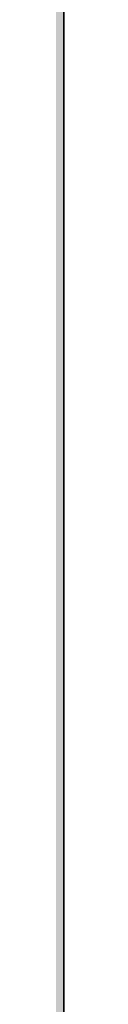
# Model space of a CAD drawing. Units: inches. Extents: x 2091 to 2899, y 967 to 2217.
# Tile 65 of 256: x 2212.1436 to 2212.1436, y 1100.4988 to 1101.1654. Entities that reach past the tile are written whole.
import ezdxf

# ---------------------------------------------------------------- set-up
doc = ezdxf.new("R2010")
doc.units = ezdxf.units.IN
doc.layers.add('A-WALL', color=7, linetype='Continuous', lineweight=35)
doc.layers.add('A-WALL-PATT', color=141, linetype='Continuous', lineweight=13, true_color=0xadddf7)

msp = doc.modelspace()

# ---------------------------------------------------------------- hatches: boundary and pattern name
at = {"layer": 'A-WALL-PATT'}
h = msp.add_hatch(color=256, dxfattribs=at)
h.dxf.hatch_style = 1
h.paths.add_polyline_path([(2212.1436, 1941.41906), (2387.6436, 1941.41906), (2387.6436, 1824.41906), (2392.1436, 1824.41906), (2392.1436, 1941.41906), (2609.6436, 1941.41906), (2609.6436, 1825.91906), (2614.1436, 1825.91906), (2614.1436, 1941.41906), (2794.1436, 1941.41906), (2794.1436, 1928.76217), (2803.1436, 1928.76217), (2803.1436, 2050.91906), (2203.1436, 2050.91906), (2203.1436, 1900.75786), (2212.1436, 1900.75786)])
h.paths.add_polyline_path([(2212.1436, 1945.91906), (2212.1436, 2041.91906), (2794.1436, 2041.91906), (2794.1436, 1945.91906), (2402.24824, 1945.91906), (2401.10243, 1945.77583), (2398.70243, 1945.77583)], flags=16)
h.paths.add_polyline_path([(2230.22986, 1948.06279), (2227.34986, 1949.50279), (2225.90986, 1951.90279), (2223.98986, 1952.86279), (2223.02986, 1955.26279), (2222.06986, 1959.58279), (2222.06986, 1963.42279), (2223.02986, 1965.66279), (2223.98986, 1965.34279), (2225.58591, 1963.86075), (2226.91153, 1964.95726), (2226.94886, 1965.93879), (2227.77832, 1966.95214), (2228.19992, 1968.8787), (2230.70986, 1964.86279), (2233.58986, 1966.30279), (2233.60731, 1966.33187), (2233.77266, 1964.9382), (2234.6338, 1963.67647), (2235.02986, 1963.90279), (2236.28203, 1965.57236), (2235.98986, 1962.94279), (2237.95451, 1957.54), (2238.38986, 1957.90279), (2239.21586, 1960.30579), (2238.65457, 1966.38496), (2238.69279, 1966.43807), (2238.84058, 1967.49971), (2238.78029, 1967.68749), (2238.88054, 1967.78676), (2238.66686, 1966.25179), (2239.21586, 1960.30579), (2238.38986, 1957.90279), (2236.94986, 1956.70279), (2234.54986, 1949.98279)], flags=0)
h.paths.add_polyline_path([(2278.01197, 1948.06279), (2276.49643, 1947.87335), (2275.84983, 1947.68861), (2274.65197, 1947.10279)], flags=0)
h.paths.add_polyline_path([(2269.85197, 1955.74279), (2268.27618, 1956.62933), (2270.8673, 1956.3484), (2269.37197, 1958.14279), (2268.71496, 1959.19233), (2270.56983, 1958.72861), (2268.58073, 1961.90609), (2270.81197, 1960.89188), (2270.81197, 1963.42279), (2271.39331, 1964.77926), (2270.29176, 1966.1562), (2271.77197, 1965.66279), (2272.14139, 1966.52476), (2273.92983, 1965.92861), (2275.63039, 1968.0543), (2276.33194, 1966.72186), (2276.52043, 1966.95214), (2276.94203, 1968.8787), (2277.73429, 1967.61108), (2278.13989, 1969.46452), (2279.65912, 1967.03374), (2280.41197, 1966.78279), (2280.9493, 1967.58879), (2281.60983, 1967.36861), (2282.13327, 1968.15376), (2282.34924, 1966.33344), (2282.34985, 1966.33259), (2283.40755, 1968.09542), (2283.71263, 1965.52402), (2284.32022, 1964.63379), (2284.51181, 1964.88924), (2284.23497, 1965.70479), (2284.50047, 1967.31896), (2284.90794, 1965.41742), (2285.39631, 1966.06858), (2285.43283, 1966.29061), (2285.47334, 1966.17128), (2286.35392, 1967.34539), (2286.22201, 1966.15817), (2287.66349, 1968.08015), (2287.71397, 1968.44279), (2288.4816, 1969.01668), (2288.57399, 1968.7289), (2288.91746, 1969.06904), (2288.60683, 1966.83761), (2288.92873, 1963.35131), (2288.93497, 1963.35679), (2288.92973, 1963.34042), (2289.01528, 1962.41387), (2290.11122, 1963.87513), (2290.13283, 1963.94261), (2290.21767, 1964.01706), (2290.11122, 1963.87513), (2289.15583, 1960.89161), (2288.59404, 1959.25723), (2288.57197, 1959.10279), (2289.53197, 1960.54279), (2290.01197, 1962.46279), (2290.19184, 1962.64266), (2289.76983, 1959.68861), (2286.88983, 1957.28861), (2284.48983, 1950.56861), (2283.31466, 1950.04631), (2283.29197, 1949.98279), (2280.29006, 1948.64861), (2281.12983, 1948.64861), (2282.56983, 1948.16861), (2283.20473, 1948.06279), (2278.97197, 1948.06279), (2276.09197, 1949.50279), (2274.65197, 1951.90279), (2272.73197, 1952.86279)], flags=0)
h.paths.add_polyline_path([(2271.15887, 1958.02177), (2272.96983, 1955.84861), (2272.00983, 1960.16861), (2272.00983, 1964.00861), (2272.62443, 1965.44266), (2274.32802, 1963.86075), (2275.65365, 1964.95726), (2275.63774, 1964.53909), (2277.41223, 1966.00689), (2277.03297, 1965.15679), (2276.82992, 1964.9756), (2276.76601, 1963.29501), (2277.44964, 1962.66022), (2279.45197, 1964.86279), (2282.33197, 1966.30279), (2283.52983, 1966.88861), (2283.29451, 1966.77095), (2283.91299, 1963.8847), (2284.89925, 1964.44827), (2284.73197, 1962.94279), (2286.69662, 1957.54), (2287.13197, 1957.90279), (2287.54191, 1959.09539), (2287.7794, 1958.44231), (2285.68274, 1956.6951), (2285.8765, 1959.79534), (2284.73197, 1962.94279), (2284.89925, 1964.44827), (2283.91299, 1963.8847), (2284.22383, 1962.43412), (2283.42436, 1963.60548), (2281.60983, 1962.56861), (2281.12983, 1960.16861), (2282.08983, 1956.32861), (2283.04983, 1952.96861), (2282.56983, 1950.56861), (2280.16983, 1948.64861), (2279.88332, 1948.79187), (2278.97197, 1948.06279), (2278.97197, 1949.02279), (2278.67231, 1949.39737), (2277.28983, 1950.08861), (2275.84983, 1952.48861), (2273.92983, 1953.44861), (2272.48983, 1954.88861), (2271.92165, 1954.88861), (2271.77197, 1955.26279)], flags=0)
h.paths.add_polyline_path([(2311.99415, 1955.74279), (2312.06272, 1955.67422), (2312.0551, 1955.7085)], flags=0)
h.paths.add_polyline_path([(2331.95615, 1963.95179), (2333.39615, 1965.39179), (2331.07715, 1963.35679), (2330.9986, 1963.11152)], flags=0)
h.paths.add_polyline_path([(2310.55415, 1954.30279), (2307.03981, 1956.27994), (2310.7629, 1955.87628), (2312.47415, 1953.82279), (2313.43415, 1951.42279), (2315.35415, 1950.46279), (2316.79415, 1948.06279), (2317.46615, 1947.72679), (2319.36869, 1947.96461), (2317.75415, 1949.98279), (2317.56953, 1950.61048), (2316.79415, 1951.90279), (2314.87415, 1952.86279), (2313.91415, 1955.26279), (2311.51415, 1958.14279), (2309.37549, 1961.55917), (2311.51415, 1960.33708), (2311.51415, 1961.98279), (2310.60467, 1963.11963), (2311.72661, 1962.47853), (2312.41833, 1964.09256), (2312.25596, 1964.29552), (2313.19415, 1963.98279), (2313.91415, 1965.66279), (2314.64678, 1965.41858), (2315.35415, 1966.30279), (2316.79415, 1967.74279), (2316.15744, 1966.9469), (2317.03411, 1965.28186), (2317.2226, 1965.51214), (2317.77705, 1968.04577), (2318.47411, 1966.72186), (2318.6626, 1966.95214), (2319.0842, 1968.8787), (2321.20705, 1965.48215), (2322.16142, 1966.9137), (2322.55415, 1966.78279), (2322.78599, 1967.13056), (2322.88165, 1966.32429), (2323.31204, 1965.72174), (2323.65129, 1965.89136), (2324.3965, 1967.13338), (2324.65694, 1964.9382), (2324.97199, 1964.47661), (2325.38728, 1967.0015), (2325.94081, 1964.41835), (2327.22893, 1966.13584), (2327.16632, 1965.57236), (2328.05914, 1966.76278), (2328.22458, 1966.24749), (2329.66797, 1967.67691), (2329.66458, 1967.68749), (2329.76482, 1967.78676), (2329.55115, 1966.25179), (2330.10015, 1960.30579), (2329.33281, 1958.07347), (2329.31306, 1957.93523), (2329.63415, 1958.20279), (2330.23415, 1959.10279), (2330.71415, 1961.02279), (2331.03415, 1961.34279), (2330.71415, 1959.10279), (2329.63415, 1958.20279), (2329.27415, 1957.66279), (2327.71211, 1956.3611), (2325.43415, 1949.98279), (2324.33377, 1949.49374), (2323.99415, 1948.54279), (2319.67415, 1946.62279), (2316.79415, 1948.06279), (2315.35415, 1950.46279), (2313.43415, 1951.42279)], flags=0)
h.paths.add_polyline_path([(2321.33568, 1947.95202), (2321.11415, 1948.06279), (2321.11415, 1949.02279), (2319.19415, 1951.42279), (2316.79415, 1959.58279), (2316.66324, 1959.58279), (2315.35415, 1958.14279), (2314.39415, 1958.14279), (2313.1483, 1958.70908), (2312.95415, 1959.58279), (2312.95415, 1960.89188), (2315.83415, 1959.58279), (2316.66324, 1959.58279), (2317.31471, 1960.29941), (2315.0302, 1962.42075), (2316.35582, 1963.51726), (2316.37234, 1963.95162), (2316.4702, 1963.86075), (2317.79582, 1964.95726), (2317.75522, 1963.88969), (2319.17515, 1965.15679), (2319.49841, 1965.88137), (2321.11415, 1965.34279), (2323.23589, 1962.37236), (2325.68635, 1963.77262), (2325.54279, 1962.48058), (2325.19878, 1963.49401), (2324.47851, 1963.08243), (2324.92601, 1960.99412), (2324.07809, 1962.23647), (2322.41479, 1961.28602), (2322.07415, 1959.58279), (2323.03415, 1955.74279), (2323.99415, 1952.38279), (2323.51415, 1949.98279), (2322.14272, 1948.88565), (2322.07415, 1948.54279)], flags=0)
h.paths.add_polyline_path([(2320.20748, 1963.33746), (2320.15415, 1963.42279), (2320.39415, 1963.54279)], flags=0)
h.paths.add_polyline_path([(2353.85053, 1965.8105), (2354.03053, 1965.7505), (2354.33053, 1966.4505), (2354.33053, 1966.9305)], flags=0)
h.paths.add_polyline_path([(2359.02058, 1969.02641), (2359.09838, 1968.90193), (2359.23353, 1969.5195), (2359.23353, 1969.9995)], flags=0)
h.paths.add_polyline_path([(2358.25669, 1966.68167), (2357.9836, 1966.34803), (2358.21127, 1966.14617), (2358.41049, 1966.38957)], flags=0)
h.paths.add_polyline_path([(2357.76847, 1966.05878), (2357.7322, 1965.10497), (2357.75105, 1965.12056), (2357.76953, 1965.6065), (2357.76953, 1966.05784)], flags=0)
h.paths.add_polyline_path([(2359.11153, 1965.3045), (2359.11153, 1964.8245), (2359.84453, 1966.4675), (2359.84453, 1966.9475)], flags=0)
h.paths.add_polyline_path([(2360.22368, 1966.62145), (2360.69853, 1969.3625), (2360.69853, 1969.8425), (2360.21053, 1967.0255), (2360.21053, 1966.6425)], flags=0)
h.paths.add_polyline_path([(2363.45053, 1967.8905), (2363.45053, 1968.3705), (2362.49053, 1966.9305), (2362.65604, 1966.69878)], flags=0)
h.paths.add_polyline_path([(2364.47552, 1966.07883), (2365.85053, 1968.3705), (2365.85053, 1968.8505), (2364.42798, 1966.47958)], flags=0)
h.paths.add_polyline_path([(2366.31353, 1965.8525), (2366.36671, 1965.69583), (2366.80253, 1968.3455), (2366.80253, 1968.8255)], flags=0)
h.paths.add_polyline_path([(2367.16531, 1965.80354), (2367.29053, 1966.9305), (2367.29053, 1967.4105), (2367.1027, 1965.72007)], flags=0)
h.paths.add_polyline_path([(2370.03653, 1959.9735), (2371.01353, 1963.0245), (2371.01353, 1963.5045), (2370.03653, 1960.4535)], flags=0)
h.paths.add_polyline_path([(2371.61053, 1960.2105), (2372.57053, 1961.6505), (2372.57053, 1962.1305), (2371.80253, 1960.9785)], flags=0)
h.paths.add_polyline_path([(2350.87367, 1956.00509), (2351.93053, 1955.8905), (2354.49053, 1953.3305), (2353.85053, 1954.9305), (2351.45053, 1957.8105), (2347.93553, 1963.4255), (2347.93553, 1963.9055), (2351.45053, 1958.2905), (2353.70507, 1955.58505), (2352.89053, 1959.2505), (2352.89053, 1959.7305), (2352.89053, 1961.92479), (2356.73053, 1959.7305), (2358.45447, 1961.62684), (2354.81053, 1965.0105), (2355.03086, 1965.28591), (2358.69109, 1961.88712), (2361.53053, 1965.0105), (2364.3765, 1966.43348), (2364.52439, 1965.18691), (2365.45447, 1963.82418), (2365.88107, 1964.06795), (2365.37053, 1966.4505), (2365.37053, 1966.9305), (2366.81053, 1960.2105), (2366.81053, 1959.7305), (2366.38871, 1952.98141), (2367.77053, 1956.8505), (2368.64123, 1957.57608), (2366.81053, 1962.6105), (2366.81053, 1963.0905), (2368.77518, 1957.68771), (2369.21053, 1958.0505), (2370.00159, 1960.35187), (2369.47523, 1966.05267), (2369.51346, 1966.10578), (2369.51417, 1966.11091), (2369.47523, 1966.53267), (2369.51346, 1966.58578), (2369.61463, 1967.31259), (2369.18253, 1968.6585), (2369.18253, 1969.1385), (2369.60096, 1967.83519), (2369.7012, 1967.93447), (2369.71795, 1968.05474), (2370.14518, 1968.37414), (2369.77871, 1968.01122), (2369.7012, 1967.45447), (2370.46816, 1968.214), (2369.67494, 1967.26577), (2369.51417, 1966.11091), (2370.03653, 1960.4535), (2370.03653, 1959.9735), (2369.44176, 1958.24319), (2370.65053, 1959.2505), (2371.04582, 1962.01756), (2371.13053, 1962.1305), (2370.65053, 1958.7705), (2367.77053, 1956.3705), (2365.37053, 1949.6505), (2362.0791, 1948.18764), (2363.45053, 1947.7305), (2361.05053, 1947.7305), (2360.09053, 1947.7305), (2357.10386, 1947.35717), (2360.09053, 1948.2105), (2358.17053, 1949.1705), (2356.73053, 1951.5705), (2354.81053, 1952.5305), (2351.93053, 1955.4105)], flags=0)
h.paths.add_polyline_path([(2361.05053, 1948.6905), (2359.13053, 1951.0905), (2356.73053, 1959.2505), (2355.77053, 1959.2505), (2352.89053, 1960.55959), (2352.89053, 1961.44479), (2355.89053, 1959.7305), (2356.73053, 1959.7305), (2356.83719, 1959.36783), (2361.53053, 1964.5305), (2363.24842, 1965.38945), (2364.92531, 1963.0418), (2362.49053, 1961.6505), (2362.06386, 1959.51717), (2362.97053, 1955.8905), (2363.93053, 1952.5305), (2363.93053, 1952.0505), (2363.45053, 1949.6505), (2361.05053, 1947.7305)], flags=0)
h.paths.add_polyline_path([(2359.13053, 1951.5705), (2359.29053, 1951.3705), (2361.05053, 1954.4505), (2361.05053, 1954.9305)], flags=0)
h.paths.add_polyline_path([(2357.21953, 1966.5455), (2356.79253, 1968.8145), (2356.79253, 1969.2945), (2357.21953, 1967.0255)], flags=0)
h.paths.add_polyline_path([(2361.05053, 1954.4505), (2361.53053, 1958.7705), (2361.53053, 1959.2505), (2361.05053, 1954.9305)], flags=0)
h.paths.add_polyline_path([(2402.54829, 1948.48608), (2402.30243, 1948.41583), (2402.59043, 1948.41583)], flags=0)
h.paths.add_polyline_path([(2394.14243, 1956.09583), (2395.68505, 1954.55321), (2396.7205, 1953.97068), (2396.06243, 1955.61583), (2395.24138, 1956.6011), (2395.8789, 1956.44171), (2395.10243, 1959.93583), (2395.10243, 1963.77583), (2396.06243, 1966.01583), (2397.02243, 1965.69583), (2398.61848, 1964.21379), (2399.94411, 1965.3103), (2399.98143, 1966.29183), (2400.81089, 1967.30518), (2401.23249, 1969.23174), (2403.53795, 1965.54301), (2403.94198, 1967.38932), (2404.70243, 1967.13583), (2405.46033, 1966.07478), (2406.62243, 1966.65583), (2406.63988, 1966.68491), (2406.80523, 1965.29124), (2406.92569, 1965.11475), (2407.34243, 1964.97583), (2407.87433, 1965.77367), (2408.1691, 1964.39805), (2409.31461, 1965.9254), (2409.21746, 1965.05105), (2409.44523, 1963.13124), (2410.30637, 1961.86951), (2410.70243, 1962.09583), (2411.44227, 1963.08228), (2411.16543, 1963.89783), (2411.61643, 1966.63976), (2411.72536, 1966.79111), (2411.87315, 1967.85275), (2411.81286, 1968.04053), (2411.91311, 1968.1398), (2411.69943, 1966.60483), (2412.24843, 1960.65883), (2413.22543, 1963.70983), (2414.3779, 1964.72116), (2414.51315, 1965.69275), (2414.45286, 1965.88053), (2414.55311, 1965.9798), (2414.3779, 1964.72116), (2414.51982, 1964.8457), (2414.36536, 1964.63111), (2414.33943, 1964.44483), (2414.88843, 1958.49883), (2414.06243, 1956.09583), (2412.62243, 1954.89583), (2410.17137, 1948.03285), (2410.01672, 1948.0844), (2405.90243, 1946.25583), (2405.90243, 1947.21583), (2405.20425, 1948.08856), (2404.22243, 1948.41583), (2403.26243, 1948.41583), (2400.38243, 1949.85583), (2399.66243, 1951.05583), (2397.98243, 1952.73583), (2397.02243, 1953.21583), (2395.68505, 1954.55321), (2392.65678, 1956.25691)], flags=0)
h.paths.add_polyline_path([(2409.08565, 1964.40744), (2409.13036, 1964.27572), (2409.26243, 1964.49583)], flags=0)
h.paths.add_polyline_path([(2397.74243, 1961.61583), (2398.70243, 1963.85583), (2399.66243, 1963.53583), (2401.42656, 1965.74099), (2401.79142, 1966.5588), (2402.07143, 1965.07083), (2402.83551, 1964.39337), (2403.2624, 1964.9149), (2403.33812, 1964.77109), (2402.61552, 1963.97622), (2402.49861, 1960.90224), (2403.543, 1959.93245), (2404.4132, 1960.88968), (2404.70243, 1962.33583), (2407.91635, 1964.17235), (2409.52021, 1961.92694), (2410.98708, 1957.89304), (2411.42243, 1958.25583), (2412.04796, 1960.07562), (2412.41034, 1959.07909), (2411.67562, 1958.46682), (2411.66243, 1958.25583), (2411.62607, 1958.42553), (2409.98243, 1957.05583), (2407.58243, 1950.33583), (2403.26243, 1948.41583), (2403.26243, 1949.37583), (2401.34243, 1951.77583), (2399.41651, 1958.32398), (2397.74243, 1959.08492), (2397.74243, 1959.97012), (2397.10243, 1960.33583), (2397.74243, 1960.04492)], flags=0)
h.paths.add_polyline_path([(2405.90243, 1952.97583), (2405.95043, 1953.40783), (2406.01672, 1953.17583)], flags=0)
h.paths.add_polyline_path([(2449.81778, 1967.11401), (2449.75232, 1967.13583), (2449.7937, 1967.0779)], flags=0)
h.paths.add_polyline_path([(2451.6977, 1966.61812), (2451.74089, 1966.69012), (2451.69205, 1966.6657)], flags=0)
h.paths.add_polyline_path([(2454.34363, 1965.73757), (2455.75232, 1967.61583), (2455.99232, 1968.09583), (2454.3645, 1965.9254)], flags=0)
h.paths.add_polyline_path([(2457.54732, 1968.86383), (2457.78732, 1969.34383), (2457.05432, 1968.79583), (2457.00762, 1968.46034)], flags=0)
h.paths.add_polyline_path([(2456.92178, 1967.85666), (2456.80224, 1968.22902), (2456.723, 1967.6598)], flags=0)
h.paths.add_polyline_path([(2457.30232, 1967.37683), (2457.54232, 1967.85683), (2456.81032, 1966.83983), (2456.74052, 1966.70022), (2456.74902, 1966.60811)], flags=0)
h.paths.add_polyline_path([(2458.27532, 1963.70983), (2458.15534, 1963.33515), (2460.35432, 1965.26483), (2460.59432, 1965.74483)], flags=0)
h.paths.add_polyline_path([(2458.39232, 1962.81583), (2458.36409, 1962.61819), (2459.59232, 1964.25583), (2459.83232, 1964.73583)], flags=0)
h.paths.add_polyline_path([(2459.35232, 1962.81583), (2459.27232, 1962.49583), (2460.07232, 1963.29583), (2460.31232, 1963.77583)], flags=0)
h.paths.add_polyline_path([(2458.68032, 1960.60783), (2458.63232, 1960.41583), (2459.59232, 1961.85583), (2459.83232, 1962.33583)], flags=0)
h.paths.add_polyline_path([(2437.83817, 1956.24265), (2439.19232, 1956.09583), (2441.35232, 1953.93583), (2440.87232, 1955.13583), (2438.47232, 1958.01583), (2438.07156, 1958.65602), (2438.71232, 1958.49583), (2440.6396, 1956.18311), (2439.91232, 1959.45583), (2439.91232, 1963.29583), (2441.35232, 1966.65583), (2441.59232, 1967.13583), (2441.11232, 1966.01583), (2442.07232, 1965.69583), (2443.98899, 1968.09167), (2444.24132, 1966.75083), (2444.9168, 1966.15192), (2445.67657, 1967.08014), (2446.25532, 1969.72483), (2446.49532, 1970.20483), (2446.28238, 1969.23174), (2447.36267, 1967.50327), (2447.72032, 1969.56783), (2447.96032, 1970.04783), (2447.48548, 1967.30678), (2448.79232, 1965.21583), (2448.47232, 1964.86383), (2448.55232, 1964.73583), (2451.45205, 1966.1857), (2451.61512, 1964.81124), (2452.30792, 1963.79617), (2453.23451, 1964.32565), (2454.07232, 1960.41583), (2453.62869, 1953.31765), (2454.79232, 1956.57583), (2455.03232, 1957.05583), (2455.71884, 1957.62793), (2453.83232, 1962.81583), (2453.94097, 1963.79362), (2453.33532, 1965.57783), (2453.82432, 1968.55083), (2454.06432, 1969.03083), (2453.57532, 1966.05783), (2454.04033, 1964.68792), (2453.83232, 1962.81583), (2455.71884, 1957.62793), (2456.36721, 1958.16824), (2457.05832, 1960.17883), (2457.29832, 1960.65883), (2456.47232, 1958.25583), (2457.71773, 1959.29367), (2457.67232, 1958.97583), (2454.88995, 1956.65719), (2453.61414, 1953.08492), (2453.59232, 1952.73583), (2453.35232, 1952.25583), (2453.3596, 1952.3722), (2452.63232, 1950.33583), (2452.39232, 1949.85583), (2449.20375, 1948.43869), (2450.71232, 1947.93583), (2448.07232, 1947.93583), (2447.11232, 1947.93583), (2444.55232, 1947.61583), (2447.1996, 1948.3722), (2445.19232, 1949.37583), (2443.75232, 1951.77583), (2441.83232, 1952.73583), (2438.95232, 1955.61583)], flags=0)
h.paths.add_polyline_path([(2443.99232, 1959.93583), (2444.04032, 1959.77263), (2444.12155, 1959.86199)], flags=0)
h.paths.add_polyline_path([(2442.91232, 1959.93583), (2443.03232, 1959.93583), (2442.44566, 1960.2025)], flags=0)
h.paths.add_polyline_path([(2444.98294, 1965.01968), (2445.27932, 1965.26483), (2445.51932, 1965.74483), (2444.994, 1965.3103)], flags=0)
h.paths.add_polyline_path([(2446.13332, 1965.02983), (2446.33037, 1965.4715), (2444.97032, 1964.25783), (2444.73032, 1963.77783)], flags=0)
h.paths.add_polyline_path([(2442.79232, 1959.45583), (2443.75232, 1959.45583), (2446.15232, 1951.29583), (2446.41232, 1951.75083), (2446.39232, 1951.77583), (2448.0806, 1954.73032), (2448.55232, 1958.97583), (2441.83232, 1965.21583), (2442.15495, 1965.61911), (2448.79232, 1959.45583), (2448.31232, 1955.13583), (2448.07232, 1954.65583), (2446.41232, 1951.75083), (2448.31232, 1949.37583), (2448.31232, 1948.41583), (2450.54089, 1950.19869), (2450.95232, 1952.25583), (2449.99232, 1955.61583), (2449.03232, 1959.45583), (2449.51232, 1961.85583), (2449.75232, 1962.33583), (2449.6749, 1961.94874), (2452.99451, 1963.84565), (2453.06441, 1963.51941), (2452.88461, 1963.78285), (2449.6749, 1961.94874), (2449.27232, 1959.93583), (2450.23232, 1956.09583), (2451.19232, 1952.73583), (2450.71232, 1950.33583), (2450.47232, 1949.85583), (2448.07232, 1947.93583), (2448.07232, 1948.53583), (2445.43232, 1949.85583), (2443.99232, 1952.25583), (2442.07232, 1953.21583), (2441.11232, 1955.61583), (2440.15232, 1959.93583), (2440.15232, 1960.65583)], flags=0)
h.paths.add_polyline_path([(2456.69232, 1966.98583), (2457.60832, 1968.08083), (2457.84832, 1968.56083), (2456.93232, 1967.46583)], flags=0)
h.paths.add_polyline_path([(2489.89657, 1966.58024), (2489.94295, 1966.18935), (2490.74749, 1967.53025), (2491.31912, 1968.95116)], flags=0)
h.paths.add_polyline_path([(2473.56247, 1956.40713), (2477.13998, 1956.01926), (2476.95533, 1956.24083), (2475.10805, 1957.28011), (2476.34749, 1956.97025), (2475.1869, 1958.82422), (2476.91912, 1958.39116), (2475.41164, 1960.79927), (2477.78749, 1959.71934), (2477.78749, 1962.25025), (2477.6374, 1962.43786), (2477.82255, 1962.33206), (2478.35912, 1963.58406), (2478.35912, 1963.67116), (2477.32435, 1964.96463), (2478.71483, 1964.50114), (2479.31912, 1965.91116), (2480.27912, 1965.59116), (2481.78397, 1967.47221), (2482.11649, 1965.70525), (2482.88056, 1965.02778), (2483.20931, 1965.42941), (2483.22017, 1965.71509), (2483.07594, 1965.98902), (2483.71176, 1966.76581), (2484.13049, 1968.67925), (2484.70212, 1970.10016), (2484.48918, 1969.12707), (2486.5029, 1965.90511), (2487.38749, 1965.61025), (2488.15342, 1966.75914), (2488.71702, 1965.97011), (2489.20009, 1966.21164), (2489.33067, 1965.11099), (2490.3939, 1963.62246), (2490.66077, 1963.77496), (2490.49391, 1964.55364), (2490.92306, 1963.92484), (2491.31912, 1964.15116), (2491.33339, 1964.17018), (2491.21049, 1964.53225), (2491.28176, 1964.96554), (2491.42579, 1964.29338), (2494.07648, 1967.82763), (2494.49792, 1966.51494), (2494.59817, 1966.61422), (2494.68949, 1967.27025), (2495.10675, 1967.5822), (2495.12984, 1967.74807), (2495.06955, 1967.93585), (2495.1698, 1968.03513), (2495.03178, 1967.04363), (2495.75382, 1967.75868), (2494.98205, 1966.68644), (2494.95612, 1966.50016), (2495.47902, 1960.83685), (2495.91049, 1962.18425), (2496.48212, 1963.60516), (2496.07269, 1962.32659), (2496.7689, 1962.93754), (2496.59912, 1962.71116), (2496.11912, 1959.35116), (2496.73287, 1960.27179), (2496.98749, 1961.29025), (2497.55912, 1962.71116), (2497.07912, 1960.79116), (2496.50749, 1959.37025), (2495.54749, 1957.93025), (2492.75884, 1955.60638), (2490.83912, 1950.23116), (2490.26749, 1948.81025), (2485.94749, 1946.89025), (2483.06749, 1948.33025), (2481.62749, 1950.73025), (2479.70749, 1951.69025), (2476.82749, 1954.57025)], flags=0)
h.paths.add_polyline_path([(2485.57697, 1948.31339), (2485.55912, 1948.31116), (2485.57876, 1948.31116)], flags=0)
h.paths.add_polyline_path([(2478.64506, 1954.55116), (2478.10904, 1956.96326), (2479.31912, 1955.51116), (2480.27912, 1953.11116), (2482.19912, 1952.15116), (2483.63912, 1949.75116), (2486.51912, 1948.31116), (2486.51912, 1949.27116), (2484.73931, 1951.49593), (2484.02749, 1950.25025), (2481.62749, 1958.41025), (2482.37515, 1959.23267), (2482.19912, 1959.83116), (2483.19757, 1960.92946), (2479.70749, 1964.17025), (2480.60336, 1965.29008), (2481.87517, 1964.10911), (2482.66639, 1964.76358), (2482.61536, 1963.4218), (2482.9892, 1963.07466), (2484.00849, 1963.98425), (2484.68361, 1965.49751), (2484.58012, 1965.40516), (2485.35727, 1967.14711), (2485.12065, 1965.7812), (2486.42749, 1963.69025), (2488.14538, 1964.5492), (2489.82227, 1962.20155), (2490.74749, 1962.73025), (2491.99966, 1964.39981), (2492.07605, 1965.08726), (2492.21289, 1964.68412), (2492.48537, 1965.04743), (2492.27912, 1963.19116), (2494.24377, 1957.78837), (2494.5625, 1958.05398), (2494.93349, 1959.13325), (2495.50512, 1960.55416), (2494.67912, 1958.15116), (2494.10749, 1956.73025), (2494.5625, 1958.05398), (2493.40854, 1957.09235), (2491.70749, 1961.77025), (2491.99966, 1964.39981), (2490.74749, 1962.73025), (2487.71203, 1960.9957), (2487.47912, 1959.83116), (2488.43912, 1955.99116), (2489.39912, 1952.63116), (2488.91912, 1950.23116), (2488.57692, 1949.9574), (2488.34749, 1948.81025), (2487.65172, 1948.25363), (2487.47912, 1948.31116), (2486.51912, 1948.31116), (2483.63912, 1949.75116), (2482.19912, 1952.15116), (2480.27912, 1953.11116), (2478.83912, 1954.55116)], flags=0)
h.paths.add_polyline_path([(2526.64825, 1966.98752), (2526.51734, 1967.03116), (2526.6001, 1966.9153)], flags=0)
h.paths.add_polyline_path([(2528.47064, 1966.44666), (2528.57449, 1966.61973), (2528.45707, 1966.56102)], flags=0)
h.paths.add_polyline_path([(2534.13334, 1967.49616), (2534.15669, 1967.54285), (2534.05984, 1967.4083)], flags=0)
h.paths.add_polyline_path([(2536.16192, 1964.0506), (2535.15734, 1962.71116), (2535.10087, 1962.31587), (2536.11734, 1963.67116), (2536.42053, 1964.27754)], flags=0)
h.paths.add_polyline_path([(2535.15734, 1959.83116), (2536.11734, 1961.27116), (2536.59734, 1962.23116), (2535.25334, 1960.21516)], flags=0)
h.paths.add_polyline_path([(2513.24904, 1956.2848), (2516.22118, 1955.96256), (2514.99734, 1957.43116), (2514.19582, 1958.71154), (2515.47734, 1958.39116), (2516.93189, 1956.64571), (2516.43734, 1958.87116), (2516.43734, 1962.71116), (2516.87269, 1963.72697), (2515.34643, 1965.6348), (2517.39734, 1964.95116), (2517.87734, 1966.07116), (2518.35734, 1967.03116), (2517.87734, 1965.91116), (2518.83734, 1965.59116), (2520.48659, 1967.65272), (2520.76634, 1966.16616), (2521.53042, 1965.48869), (2521.78144, 1965.79537), (2521.80091, 1966.30727), (2521.4778, 1966.92094), (2521.24634, 1967.12616), (2521.1777, 1967.49091), (2521.4778, 1966.92094), (2522.01042, 1966.44869), (2522.25739, 1966.75042), (2522.78034, 1969.14016), (2523.26034, 1970.10016), (2523.0474, 1969.12707), (2524.67313, 1966.5259), (2526.03734, 1966.07116), (2526.79524, 1965.01011), (2527.97707, 1965.60102), (2528.14014, 1964.22657), (2528.66459, 1963.45816), (2529.38862, 1963.87189), (2529.32967, 1964.14699), (2529.48128, 1963.92484), (2529.87734, 1964.15116), (2529.98401, 1964.29338), (2529.78905, 1965.20318), (2530.0624, 1964.3979), (2532.80248, 1968.05135), (2533.14777, 1966.97585), (2533.24802, 1967.07513), (2533.33934, 1967.73116), (2533.67285, 1967.98049), (2533.72802, 1968.03513), (2533.51434, 1966.50016), (2534.02472, 1960.9725), (2534.56034, 1962.64516), (2535.04034, 1963.60516), (2534.06334, 1960.55416), (2533.23734, 1958.15116), (2534.28815, 1959.02684), (2534.19734, 1958.39116), (2531.5126, 1956.15387), (2529.39734, 1950.23116), (2528.91734, 1949.27116), (2526.44877, 1948.17402), (2527.47734, 1947.83116), (2530.35734, 1947.35116), (2524.59734, 1947.35116), (2521.71734, 1948.79116), (2520.27734, 1951.19116), (2518.35734, 1952.15116), (2515.47734, 1955.03116)], flags=0)
h.paths.add_polyline_path([(2523.93476, 1967.19031), (2523.61951, 1966.48369), (2523.7705, 1966.24211)], flags=0)
h.paths.add_polyline_path([(2518.83734, 1953.11116), (2517.87734, 1955.51116), (2516.88498, 1959.97678), (2516.91734, 1959.96207), (2516.91734, 1962.02545), (2520.75734, 1959.83116), (2522.02495, 1961.22553), (2518.35734, 1964.63116), (2519.00259, 1965.43772), (2520.43339, 1964.10911), (2521.30112, 1964.82687), (2521.24516, 1963.35533), (2525.63831, 1959.27598), (2526.03734, 1961.27116), (2529.39734, 1963.19116), (2530.64952, 1964.86073), (2530.66472, 1964.99755), (2530.69196, 1964.91731), (2531.08778, 1965.44507), (2530.94599, 1964.16894), (2530.69196, 1964.91731), (2529.39734, 1963.19116), (2526.3625, 1961.45697), (2526.03734, 1959.83116), (2526.99734, 1955.99116), (2527.95734, 1952.63116), (2527.47734, 1950.23116), (2527.13449, 1949.95687), (2526.97393, 1949.15409), (2526.69734, 1949.03116), (2524.59734, 1947.35116), (2524.59734, 1948.31116), (2524.27734, 1948.71116), (2522.19734, 1949.75116), (2520.75734, 1952.15116)], flags=0)
h.paths.add_polyline_path([(2520.27734, 1958.87116), (2520.85334, 1959.50476), (2523.15734, 1951.67116), (2524.61389, 1954.22013), (2524.59734, 1954.07116), (2522.67734, 1950.71116)], flags=0)
h.paths.add_polyline_path([(2559.37091, 1966.31116), (2559.39841, 1966.32491), (2559.40194, 1966.3453)], flags=0)
h.paths.add_polyline_path([(2549.77091, 1957.19116), (2552.65091, 1954.31116), (2552.13399, 1955.60347), (2550.61091, 1957.43116), (2547.09591, 1963.04616), (2545.77591, 1965.20616), (2549.29091, 1959.59116), (2551.69091, 1956.71116), (2550.79293, 1960.75206), (2550.73091, 1960.78025), (2550.73091, 1964.87116), (2551.69091, 1967.11116), (2552.65091, 1966.79116), (2554.24696, 1965.30911), (2555.03425, 1965.96034), (2555.58167, 1966.64461), (2555.60991, 1967.38716), (2556.43937, 1968.40051), (2556.86097, 1970.32707), (2559.37091, 1966.31116), (2560.69091, 1964.15116), (2562.40881, 1965.01011), (2561.65091, 1966.07116), (2560.33091, 1968.23116), (2561.7585, 1966.23254), (2562.34721, 1967.11561), (2562.43371, 1966.38657), (2563.1278, 1965.3696), (2563.57091, 1965.59116), (2563.58836, 1965.62024), (2563.36254, 1967.52354), (2563.72249, 1965.84379), (2565.06, 1968.07298), (2564.73286, 1965.12872), (2565.11758, 1963.33338), (2567.44462, 1966.43611), (2567.31561, 1967.83333), (2567.35384, 1967.88644), (2567.50163, 1968.94807), (2567.44134, 1969.13585), (2567.54159, 1969.23513), (2567.32791, 1967.70016), (2567.87691, 1961.75416), (2568.74669, 1964.47033), (2568.63561, 1965.67333), (2568.67384, 1965.72644), (2568.82163, 1966.78807), (2568.76134, 1966.97585), (2568.86159, 1967.07513), (2568.64791, 1965.54016), (2568.72613, 1964.69303), (2568.85391, 1964.80516), (2568.74669, 1964.47033), (2568.81724, 1963.70626), (2568.97091, 1963.91116), (2568.86607, 1963.17731), (2569.19691, 1959.59416), (2568.37091, 1957.19116), (2566.93091, 1955.99116), (2564.62027, 1949.52137), (2564.65091, 1949.51116), (2564.61662, 1949.51116), (2564.53091, 1949.27116), (2560.21091, 1947.35116), (2557.33091, 1948.79116), (2556.0452, 1950.93402), (2556.01091, 1950.95116), (2555.85662, 1951.2083), (2553.97091, 1952.15116), (2551.09091, 1955.03116), (2546.65014, 1957.52951)], flags=0)
h.paths.add_polyline_path([(2567.02579, 1959.33023), (2567.03501, 1959.30489), (2567.05091, 1959.35116)], flags=0)
h.paths.add_polyline_path([(2551.96829, 1962.51837), (2553.01091, 1964.95116), (2553.97091, 1964.63116), (2555.56696, 1963.14911), (2556.89258, 1964.24563), (2556.92991, 1965.22716), (2557.14398, 1965.48869), (2556.42007, 1966.13056), (2556.39142, 1966.10499), (2556.37991, 1966.16616), (2556.42007, 1966.13056), (2556.95191, 1966.60516), (2557.09214, 1966.91948), (2557.57087, 1966.01023), (2557.75937, 1966.24051), (2557.41791, 1964.68016), (2556.89258, 1964.24563), (2556.80709, 1961.99757), (2560.69091, 1958.39116), (2560.63553, 1957.8927), (2560.81091, 1957.19116), (2561.77091, 1953.83116), (2561.29091, 1951.43116), (2559.11042, 1949.68677), (2559.15648, 1949.62919), (2563.02652, 1951.34921), (2562.61091, 1949.27116), (2560.21091, 1947.35116), (2560.21091, 1948.31116), (2559.25091, 1949.51116), (2558.89091, 1949.51116), (2558.89091, 1949.96116), (2558.29091, 1950.71116), (2558.0537, 1951.51767), (2556.97091, 1952.87116), (2555.06788, 1959.34146), (2552.05091, 1961.06545), (2552.05091, 1962.47116)], flags=0)
h.paths.add_polyline_path([(2588.33005, 1958.39116), (2588.61025, 1958.11096), (2588.55336, 1958.36695)], flags=0)
h.paths.add_polyline_path([(2594.74545, 1950.49309), (2593.95753, 1953.17202), (2593.13005, 1954.55116), (2591.21005, 1955.51116), (2590.25005, 1957.91116), (2588.30903, 1960.24038), (2586.17731, 1961.20935), (2587.85005, 1960.79116), (2587.25342, 1961.74425), (2588.44131, 1961.06545), (2588.44131, 1962.65553), (2588.42168, 1962.66535), (2588.44131, 1962.71116), (2586.91404, 1964.62026), (2588.87709, 1963.72796), (2589.29005, 1964.69154), (2589.29005, 1966.07116), (2590.25005, 1968.31116), (2591.21005, 1967.99116), (2592.8061, 1966.50911), (2594.13172, 1967.60563), (2594.16905, 1968.58716), (2594.99851, 1969.60051), (2595.4201, 1971.52707), (2597.93005, 1967.51116), (2600.81005, 1968.95116), (2600.8275, 1968.98024), (2600.99285, 1967.58657), (2601.85399, 1966.32484), (2602.10714, 1966.4695), (2602.23635, 1967.25507), (2602.35672, 1966.69338), (2603.50222, 1968.22073), (2603.21005, 1965.59116), (2605.1747, 1960.18837), (2605.50689, 1960.4652), (2605.02602, 1965.67333), (2605.06425, 1965.72644), (2605.21203, 1966.78807), (2605.15174, 1966.97585), (2605.25199, 1967.07513), (2605.34331, 1967.73116), (2605.9529, 1968.1869), (2605.87475, 1969.03333), (2605.91298, 1969.08644), (2606.06077, 1970.14807), (2606.00048, 1970.33585), (2606.10073, 1970.43513), (2605.88705, 1968.90016), (2606.43605, 1962.95416), (2605.61005, 1960.55116), (2605.99704, 1960.87365), (2606.56431, 1962.64516), (2608.24149, 1964.11694), (2608.01005, 1963.19116), (2607.05005, 1961.75116), (2606.63149, 1961.40236), (2606.20131, 1958.39116), (2603.32131, 1955.99116), (2600.92131, 1949.27116), (2596.60131, 1947.35116), (2593.72131, 1948.79116), (2592.85731, 1950.23116), (2592.65005, 1950.23116)], flags=0)
h.paths.add_polyline_path([(2596.60131, 1947.35116), (2596.60131, 1948.31116), (2594.68131, 1950.71116), (2596.15495, 1953.29003), (2595.53005, 1954.07116), (2593.19923, 1961.99596), (2592.65134, 1962.50471), (2591.78015, 1963.00253), (2593.28299, 1964.24563), (2593.32031, 1965.22716), (2594.14977, 1966.24051), (2594.57137, 1968.16707), (2596.18265, 1965.58902), (2596.95127, 1966.43451), (2598.04131, 1966.07116), (2598.79921, 1965.01011), (2599.96131, 1965.59116), (2599.97876, 1965.62024), (2600.14411, 1964.22657), (2601.00526, 1962.96484), (2601.40131, 1963.19116), (2602.65349, 1964.86073), (2602.36131, 1962.23116), (2603.79275, 1958.29472), (2601.97764, 1953.21243), (2601.94621, 1952.70945), (2599.46876, 1951.60836), (2599.00131, 1949.27116)], flags=0)
h.paths.add_polyline_path([(2597.56131, 1958.87116), (2597.67097, 1959.41942), (2597.59505, 1958.7362)], flags=0)
h.paths.add_polyline_path([(2623.6663, 1961.25438), (2625.51916, 1960.79116), (2624.96554, 1961.67553), (2627.19916, 1960.66025), (2627.19916, 1961.15116), (2626.95916, 1962.23116), (2626.95916, 1963.49116), (2625.58232, 1965.21221), (2626.95916, 1964.42545), (2626.95916, 1965.83116), (2626.86916, 1965.86116), (2627.91916, 1968.31116), (2628.87916, 1967.99116), (2630.47521, 1966.50911), (2631.80084, 1967.60563), (2631.83816, 1968.58716), (2632.66762, 1969.60051), (2633.08922, 1971.52707), (2635.59916, 1967.51116), (2638.47916, 1968.95116), (2638.49661, 1968.98024), (2638.66196, 1967.58657), (2639.17627, 1966.83301), (2639.78022, 1967.83958), (2640.02583, 1966.69338), (2641.17134, 1968.22073), (2640.87916, 1965.59116), (2641.11426, 1964.94463), (2641.41134, 1965.34073), (2641.3081, 1964.41159), (2642.84381, 1960.18837), (2643.27916, 1960.55116), (2644.08474, 1962.89474), (2643.78387, 1966.15333), (2643.80683, 1966.18524), (2643.60068, 1968.41805), (2643.52281, 1968.66058), (2643.72988, 1970.14807), (2643.66959, 1970.33585), (2643.76984, 1970.43513), (2643.55616, 1968.90016), (2643.60068, 1968.41805), (2643.90959, 1967.45585), (2644.00984, 1967.55513), (2643.81174, 1966.13208), (2644.10516, 1962.95416), (2644.23877, 1961.35084), (2644.71916, 1961.75116), (2645.03285, 1962.2217), (2645.32216, 1963.12516), (2646.07642, 1963.78705), (2645.03285, 1962.2217), (2644.34516, 1960.07416), (2643.51916, 1957.67116), (2642.07916, 1956.47116), (2639.71961, 1949.86442), (2639.87553, 1949.83843), (2635.35916, 1947.83116), (2632.47916, 1949.27116), (2631.03916, 1951.67116), (2629.11916, 1952.63116), (2628.15916, 1955.03116), (2625.75916, 1957.91116)], flags=0)
h.paths.add_polyline_path([(2627.81631, 1956.57402), (2627.37371, 1958.56571), (2626.37631, 1959.76259), (2627.19916, 1959.35116), (2627.37371, 1958.56571), (2627.91916, 1957.91116), (2628.87916, 1955.51116), (2630.79916, 1954.55116), (2632.23916, 1952.15116), (2633.31502, 1951.61323), (2631.03916, 1959.35116), (2631.49783, 1959.85569), (2630.79916, 1962.23116), (2631.44987, 1962.94694), (2630.71521, 1963.62911), (2632.04084, 1964.72563), (2632.07816, 1965.70716), (2632.29224, 1965.96869), (2631.70534, 1966.48907), (2633.13644, 1967.76614), (2633.32922, 1968.64707), (2634.67472, 1966.49427), (2635.20847, 1967.08139), (2636.79916, 1966.55116), (2637.6764, 1967.86702), (2638.99395, 1966.02246), (2639.70534, 1966.42898), (2641.11916, 1959.83116), (2640.93007, 1956.80571), (2639.43916, 1952.63116), (2638.22746, 1952.09262), (2637.75916, 1949.75116), (2635.35916, 1947.83116), (2635.35916, 1948.79116), (2633.43916, 1951.19116), (2633.31502, 1951.61323), (2632.23916, 1952.15116), (2630.79916, 1954.55116), (2628.87916, 1955.51116)], flags=0)
h.paths.add_polyline_path([(2637.75916, 1953.83116), (2637.27916, 1955.51116), (2636.31916, 1959.35116), (2636.79916, 1961.75116), (2639.23395, 1963.14246), (2637.55706, 1965.49011), (2638.73889, 1966.08102), (2638.90196, 1964.70657), (2639.7631, 1963.44484), (2636.79916, 1961.75116), (2636.5325, 1960.41783), (2637.03916, 1958.39116), (2637.99916, 1955.03116)], flags=0)
h.paths.add_polyline_path([(2668.56741, 1951.43116), (2667.60741, 1953.83116), (2665.20741, 1956.71116), (2662.2939, 1961.36531), (2665.44741, 1959.59116), (2666.64741, 1958.39116), (2666.64741, 1959.97516), (2666.05832, 1960.68207), (2666.64741, 1960.34545), (2666.64741, 1961.99116), (2666.70009, 1962.11409), (2666.40741, 1963.43116), (2666.40741, 1967.27116), (2667.36741, 1969.51116), (2668.32741, 1969.19116), (2669.92346, 1967.70911), (2671.24908, 1968.80563), (2671.28641, 1969.78716), (2672.11587, 1970.80051), (2672.53746, 1972.72707), (2675.04741, 1968.71116), (2677.92741, 1970.15116), (2677.94486, 1970.18024), (2678.11021, 1968.78657), (2678.97135, 1967.52484), (2679.36741, 1967.75116), (2680.61958, 1969.42073), (2680.32741, 1966.79116), (2682.29206, 1961.38837), (2682.72741, 1961.75116), (2683.35831, 1963.58657), (2683.23211, 1964.95333), (2683.27034, 1965.00644), (2683.39322, 1965.88914), (2683.35997, 1966.24921), (2683.35784, 1966.25585), (2683.35923, 1966.25723), (2682.99211, 1970.23333), (2683.03034, 1970.28644), (2683.17812, 1971.34807), (2683.11784, 1971.53585), (2683.21808, 1971.63513), (2683.00441, 1970.10016), (2683.35923, 1966.25723), (2683.45808, 1966.35513), (2683.39322, 1965.88914), (2683.41391, 1965.66502), (2684.42381, 1966.87227), (2683.55341, 1964.15416), (2683.35831, 1963.58657), (2683.79341, 1958.87416), (2682.96741, 1956.47116), (2681.52741, 1955.27116), (2680.10923, 1951.30025), (2680.08493, 1950.91157), (2679.97685, 1950.92959), (2679.12741, 1948.55116), (2674.80741, 1946.63116), (2671.92741, 1948.07116), (2670.48741, 1950.47116)], flags=0)
h.paths.add_polyline_path([(2671.93568, 1953.22702), (2671.68741, 1953.35116), (2670.24741, 1955.75116), (2668.32741, 1956.71116), (2667.35674, 1959.13783), (2669.52741, 1958.15116), (2670.48741, 1958.15116), (2671.47941, 1959.24236), (2670.6844, 1961.94538), (2668.8896, 1963.61198), (2667.30741, 1964.33116), (2668.56741, 1963.91116), (2668.83094, 1964.24057), (2670.24741, 1963.43116), (2672.42214, 1965.82337), (2672.77746, 1967.44707), (2673.23407, 1966.71649), (2674.41192, 1968.01212), (2673.98056, 1965.52211), (2675.28741, 1963.43116), (2675.55407, 1963.56449), (2675.93241, 1965.45616), (2676.24741, 1965.35116), (2677.0053, 1964.29011), (2678.16741, 1964.87116), (2679.60741, 1967.27116), (2680.32741, 1963.91116), (2680.30655, 1963.57748), (2680.34724, 1963.45761), (2680.85958, 1964.14073), (2680.56741, 1961.51116), (2681.10362, 1960.03657), (2678.88741, 1953.83116), (2677.09248, 1953.03341), (2677.68741, 1950.95116), (2677.20741, 1948.55116), (2674.80741, 1946.63116), (2674.80741, 1947.59116), (2672.88741, 1949.99116)], flags=0)
h.paths.add_polyline_path([(2673.98455, 1951.91116), (2674.56741, 1952.93116), (2674.56741, 1951.91116), (2676.96741, 1953.83116), (2677.44741, 1956.23116), (2676.48741, 1959.59116), (2676.24741, 1960.55116), (2679.72959, 1962.54098), (2680.05927, 1961.00248), (2679.21135, 1962.24484), (2676.24741, 1960.55116), (2676.48741, 1959.59116), (2677.44741, 1956.23116), (2676.96741, 1953.83116), (2674.56741, 1951.91116)], flags=0)
h.paths.add_polyline_path([(2707.47928, 1952.81465), (2706.51928, 1955.21465), (2705.55928, 1959.53465), (2705.55928, 1963.37465), (2706.51928, 1965.61465), (2707.47928, 1965.29465), (2709.07533, 1963.81261), (2710.40096, 1964.90912), (2710.43828, 1965.89065), (2711.26774, 1966.904), (2711.68934, 1968.83056), (2714.19928, 1964.81465), (2717.07928, 1966.25465), (2717.09673, 1966.28373), (2717.26208, 1964.89006), (2718.12322, 1963.62833), (2718.51928, 1963.85465), (2719.77146, 1965.52422), (2719.47928, 1962.89465), (2721.44393, 1957.49186), (2721.87928, 1957.85465), (2722.70528, 1960.25765), (2722.14399, 1966.33682), (2722.18221, 1966.38993), (2722.33, 1967.45157), (2722.26971, 1967.63934), (2722.36996, 1967.73862), (2722.15628, 1966.20365), (2722.70528, 1960.25765), (2721.87928, 1957.85465), (2720.43928, 1956.65465), (2718.03928, 1949.93465), (2713.71928, 1948.01465), (2710.83928, 1949.45465), (2709.39928, 1951.85465)], flags=0)
h.paths.add_polyline_path([(2749.30123, 1952.81465), (2748.34123, 1955.21465), (2747.38123, 1959.53465), (2747.38123, 1963.37465), (2748.34123, 1965.61465), (2749.30123, 1965.29465), (2750.89728, 1963.81261), (2752.2229, 1964.90912), (2752.26023, 1965.89065), (2753.08969, 1966.904), (2753.51129, 1968.83056), (2756.02123, 1964.81465), (2758.90123, 1966.25465), (2758.91868, 1966.28373), (2759.08403, 1964.89006), (2759.94517, 1963.62833), (2760.34123, 1963.85465), (2761.5934, 1965.52422), (2761.30123, 1962.89465), (2763.26588, 1957.49186), (2763.70123, 1957.85465), (2764.52723, 1960.25765), (2763.96594, 1966.33682), (2764.00416, 1966.38993), (2764.15195, 1967.45157), (2764.09166, 1967.63934), (2764.19191, 1967.73862), (2763.97823, 1966.20365), (2764.52723, 1960.25765), (2763.70123, 1957.85465), (2762.26123, 1956.65465), (2759.86123, 1949.93465), (2755.54123, 1948.01465), (2752.66123, 1949.45465), (2751.22123, 1951.85465)], flags=0)
h.paths.add_polyline_path([(2212.1436, 1819.93451), (2203.1436, 1819.93451), (2203.1436, 1739.97955), (2212.1436, 1739.97955), (2212.1436, 1780.91906), (2392.1436, 1780.91906), (2392.1436, 1783.91906), (2212.1436, 1783.91906)])
h.paths.add_polyline_path([(2803.1436, 1847.93882), (2794.1436, 1847.93882), (2794.1436, 1785.41906), (2609.6436, 1785.41906), (2493.87561, 1785.41906), (2493.87561, 1780.91906), (2609.6436, 1780.91906), (2794.1436, 1780.91906), (2794.1436, 1696.91906), (2609.37561, 1696.91906), (2609.37561, 1742.91906), (2604.87561, 1742.91906), (2604.87561, 1644.41906), (2609.37561, 1644.41906), (2609.37561, 1692.41906), (2794.1436, 1692.41906), (2794.1436, 1668.16474), (2803.1436, 1668.16474)])
h.paths.add_polyline_path([(2392.1436, 1740.41906), (2387.6436, 1740.41906), (2387.6436, 1629.41906), (2212.1436, 1629.41906), (2212.1436, 1659.1562), (2203.1436, 1659.1562), (2203.1436, 1494.08944), (2212.1436, 1494.08944), (2212.1436, 1627.91906), (2392.1436, 1627.91906)])
h.paths.add_polyline_path([(2457.87561, 1780.91906), (2453.37561, 1780.91906), (2453.37561, 1644.41906), (2568.87561, 1644.41906), (2568.87561, 1648.91906), (2457.87561, 1648.91906)])
h.paths.add_polyline_path([(2545.1436, 1591.91906), (2540.6436, 1591.91906), (2540.6436, 1567.91906), (2468.6436, 1567.91906), (2468.6436, 1627.91906), (2509.1436, 1627.91906), (2509.1436, 1632.41906), (2464.1436, 1632.41906), (2464.1436, 1563.41906), (2545.1436, 1563.41906)])
h.paths.add_polyline_path([(2268.6436, 1555.91906), (2212.1436, 1555.91906), (2212.1436, 1551.41906), (2268.6436, 1551.41906)], flags=17)
h.paths.add_polyline_path([(2212.1436, 1413.26609), (2203.1436, 1413.26609), (2203.1436, 1233.0704), (2212.1436, 1233.0704)])
h.paths.add_polyline_path([(2267.6436, 1351.91906), (2212.1436, 1351.91906), (2212.1436, 1347.41906), (2267.6436, 1347.41906)], flags=17)
h.paths.add_polyline_path([(2456.6436, 1489.41906), (2452.1436, 1489.41906), (2452.1436, 1351.91906), (2312.6436, 1351.91906), (2312.6436, 1347.41906), (2456.6436, 1347.41906)])
h.paths.add_polyline_path([(2472.37017, 1455.41906), (2467.87017, 1455.41906), (2467.87017, 1347.41906), (2472.37017, 1347.41906)])
h.paths.add_polyline_path([(2794.1436, 1351.91906), (2543.37017, 1351.91906), (2543.37017, 1347.41906), (2794.1436, 1347.41906)], flags=17)
h.paths.add_polyline_path([(2312.6436, 1347.41906), (2308.1436, 1347.41906), (2308.1436, 1302.16179), (2308.34197, 1302.16433), (2308.1436, 1298.16925), (2308.1436, 1275.41906), (2212.1436, 1275.41906), (2212.1436, 1270.91906), (2312.6436, 1270.91906)], flags=17)
h.paths.add_polyline_path([(2212.1436, 1152.24706), (2203.1436, 1152.24706), (2203.1436, 1090.91906), (2803.1436, 1090.91906), (2803.1436, 1392.71355), (2794.1436, 1392.71355), (2794.1436, 1143.41906), (2548.03245, 1143.41906), (2548.03245, 1138.91906), (2794.1436, 1138.91906), (2794.1436, 1099.91906), (2212.1436, 1099.91906)])
h.paths.add_polyline_path([(2471.53245, 1266.32853, 0.031658), (2467.03245, 1269.94579), (2467.03245, 1143.41906), (2471.53245, 1143.41906), (2471.53245, 1148.81906)], flags=17)
h.paths.add_polyline_path([(2803.1436, 1587.34139), (2794.1436, 1587.34139), (2794.1436, 1473.5369), (2803.1436, 1473.5369)])
h.paths.add_polyline_path([(2794.1436, 1536.41906), (2651.1436, 1536.41906), (2651.1436, 1531.91906), (2794.1436, 1531.91906)])
h.paths.add_polyline_path([(2614.1436, 1620.41906), (2609.6436, 1620.41906), (2609.6436, 1536.41906), (2614.1436, 1536.41906)])
h.paths.add_polyline_path([(2271.08273, 1964.31724), (2776.85297, 1964.31724), (2776.85297, 2037.16962), (2271.08273, 2037.16962)], flags=8)
h.paths.add_polyline_path([(2380.64929, 1536.82414), (2461.04081, 1536.82414), (2461.04081, 1554.65259), (2380.64929, 1554.65259)], flags=9)
h.paths.add_polyline_path([(2203.65504, 1608.81531), (2316.11844, 1608.81531), (2316.11844, 1621.91836), (2203.65504, 1621.91836)], flags=24)
h.paths.add_polyline_path([(2212.67726, 1313.5041), (2282.59152, 1313.5041), (2282.59152, 1322.74524), (2212.67726, 1322.74524)], flags=24)
h.paths.add_polyline_path([(2457.11198, 1114.77857), (2558.48158, 1114.77857), (2558.48158, 1142.21968), (2457.11198, 1142.21968)], flags=25)
h.paths.add_polyline_path([(2473.44234, 1273.01007), (2604.64123, 1273.01007), (2604.64123, 1318.34693), (2473.44234, 1318.34693)], flags=25)
h.paths.add_polyline_path([(2638.8763, 1626.97743), (2684.25037, 1627.97674), (2684.03848, 1637.59749), (2638.66442, 1636.59819)], flags=9)
h.paths.add_polyline_path([(2537.59055, 1453.79345), (2628.38955, 1453.79345), (2628.38955, 1475.34481), (2537.59055, 1475.34481)], flags=9)
h.paths.add_polyline_path([(2504.13764, 1714.6324), (2554.64719, 1714.6324), (2554.64719, 1730.23771), (2504.13764, 1730.23771)], flags=25)
h.paths.add_polyline_path([(2487.50118, 1575.65187), (2535.09712, 1575.65187), (2535.09712, 1598.37765), (2487.50118, 1598.37765)], flags=25)
h.paths.add_polyline_path([(2709.0994, 1735.71028), (2740.0166, 1735.71028), (2740.0166, 1749.93764), (2709.0994, 1749.93764)], flags=25)
h.paths.add_polyline_path([(2442.43842, 1792.17166), (2564.72884, 1792.17166), (2564.72884, 1842.00016), (2442.43842, 1842.00016)], flags=9)
h.paths.add_polyline_path([(2655.8158, 1809.64408), (2789.52014, 1806.6938), (2790.08498, 1832.29164), (2656.38064, 1835.24192)], flags=25)
h.paths.add_polyline_path([(2234.8427, 1797.72014), (2368.59285, 1794.76885), (2369.16072, 1820.50413), (2235.41056, 1823.45542)], flags=9)
h.paths.add_polyline_path([(2245.13847, 1644.00633), (2398.42773, 1640.6239), (2398.99484, 1666.32482), (2245.70557, 1669.70725)], flags=9)
h.paths.add_polyline_path([(2306.14285, 1431.16852), (2413.76831, 1428.79369), (2414.33315, 1454.39153), (2306.70768, 1456.76636)], flags=9)
h.paths.add_polyline_path([(2306.83458, 1458.23314), (2393.38048, 1456.32345), (2393.93281, 1481.35436), (2307.38691, 1483.26405)], flags=9)

# ---------------------------------------------------------------- linework, layer by layer
at = {"layer": 'A-WALL'}
msp.add_line((2212.1436, 1099.91906), (2212.1436, 1627.91906), dxfattribs=at)

doc.saveas('drawing.dxf')
